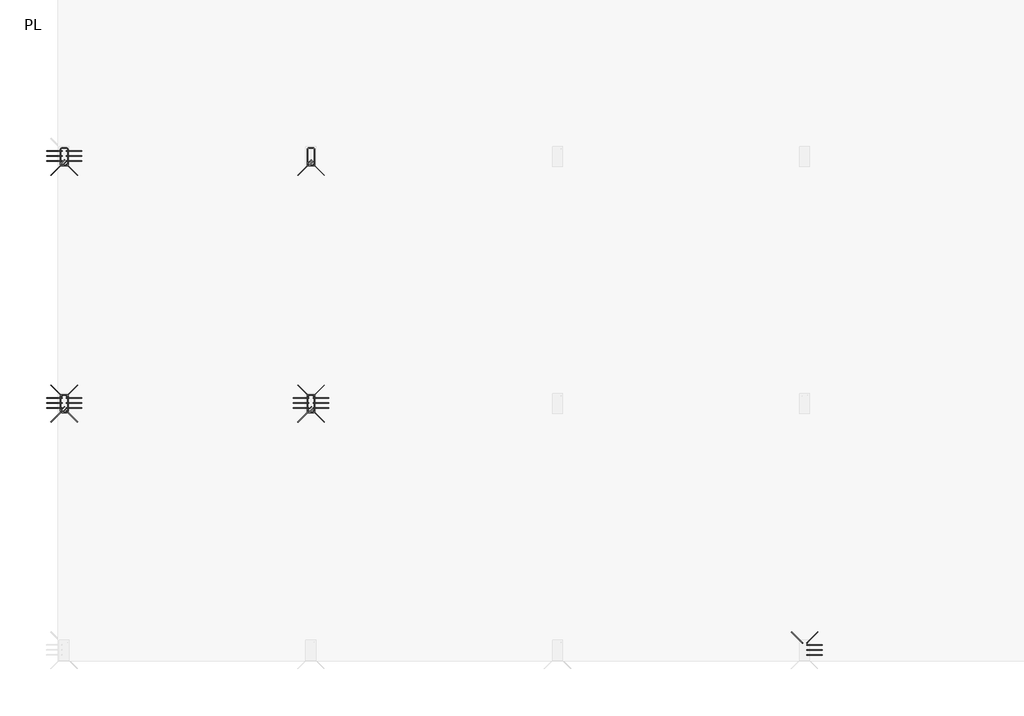
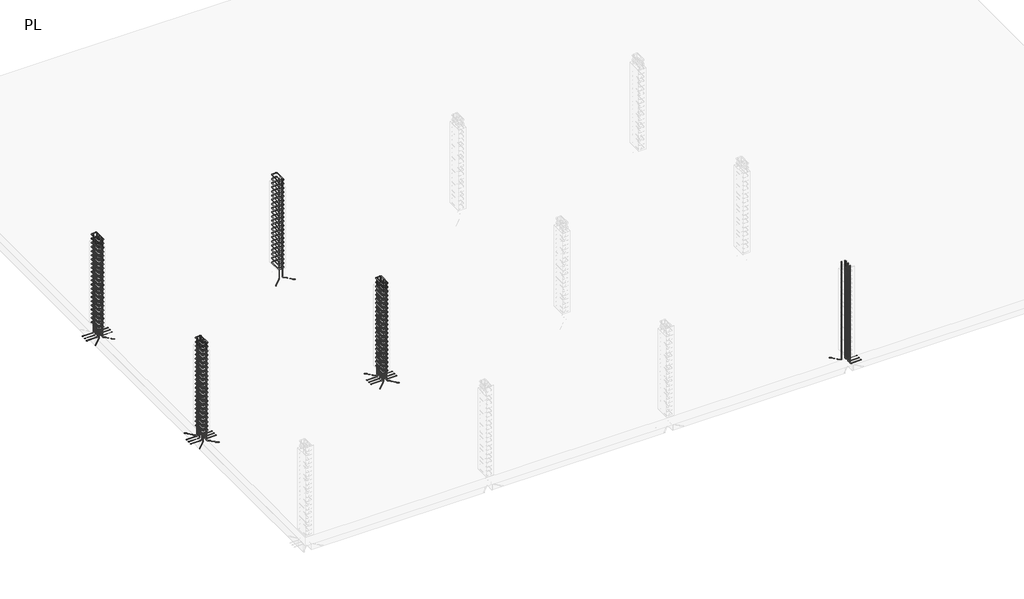
# One storey, part 4 of 10: 25 reinforcing bars.
"""IFC4 building model written with IfcOpenShell, lengths in millimetres."""

from ifc_helpers import new_model, si_unit, point, frame, origin, place, context, project, spatial, polyline, circle_curve, trimmed, segment, composite_curve, source, transform, mapped, element, save
from ifc_brep_helpers import swept_disk

model = new_model("IFC4")

# Units and contexts
model_context = context("Model", 3, world=origin())
ifc_project = project(units=[si_unit("LENGTHUNIT", "METRE", prefix="MILLI")], contexts=[model_context])

# Site, building, storey
site = spatial("IfcSite", under=ifc_project)
building = spatial("IfcBuilding", under=site)
storey = spatial("IfcBuildingStorey", under=building, Name="PL", Elevation=271.0)

# Reinforcing bars
placement = place(None, origin())
reinforcing_bar_shape = source(origin(), model_context, "Body", "SolidModel", [
    swept_disk(composite_curve([segment(polyline([(-16703.4864005, -8162.2223078, 301.0), (-16791.1676414, -8249.9035486, 301.0)]), True, "CONTINUOUS"), segment(trimmed(circle_curve(frame((-16769.9544379, -8271.1167521, 301.0), z_axis=(0.0, 0.0, 1.0), x_axis=(-21.21320349999951, 21.213203500001327, 0.0)), 30.0), [point((-16791.1676414, -8249.9035486, 301.0))], [point((-16769.9544379, -8301.1167521, 301.0))], True, "CARTESIAN"), True, "CONTINUOUS"), segment(polyline([(-16769.9544379, -8301.1167521, 301.0), (-16651.9544379, -8301.1167521, 301.0)]), True, "CONTINUOUS"), segment(trimmed(circle_curve(frame((-16651.9544379, -8271.1167521, 301.0), z_axis=(0.0, 0.0, 1.0), x_axis=(0.0, -30.0, 0.0)), 30.0), [point((-16651.9544379, -8301.1167521, 301.0))], [point((-16621.9544379, -8271.1167521, 301.0))], True, "CARTESIAN"), True, "CONTINUOUS"), segment(polyline([(-16621.9544379, -8271.1167521, 301.0), (-16621.9544379, -7903.1167521, 301.0)]), True, "CONTINUOUS"), segment(trimmed(circle_curve(frame((-16651.8864962, -7903.1167521, 298.9821084), z_axis=(-0.06726305234213417, 0.0, 0.9977352764083365), x_axis=(29.93205830000079, 0.0, 2.0178915999999845)), 30.0), [point((-16621.9544379, -7903.1167521, 301.0))], [point((-16651.8864962, -7873.1167521, 298.9821084))], True, "CARTESIAN"), True, "CONTINUOUS"), segment(polyline([(-16651.8864962, -7873.1167521, 298.9821084), (-16770.0223796, -7873.1167521, 291.0178916)]), True, "CONTINUOUS"), segment(trimmed(circle_curve(frame((-16770.0223796, -7903.1167521, 291.0178916), z_axis=(-0.06726305234213417, 0.0, 0.9977352764083365), x_axis=(0.0, 30.0, 0.0)), 30.0), [point((-16770.0223796, -7873.1167521, 291.0178916))], [point((-16799.9544379, -7903.1167521, 289.0))], True, "CARTESIAN"), True, "CONTINUOUS"), segment(polyline([(-16799.9544379, -7903.1167521, 289.0), (-16799.9544379, -8271.1167521, 289.0)]), True, "CONTINUOUS"), segment(trimmed(circle_curve(frame((-16769.9544379, -8271.1167521, 289.0), z_axis=(0.0, 0.0, 1.0), x_axis=(-30.0, 0.0, 0.0)), 30.0), [point((-16799.9544379, -8271.1167521, 289.0))], [point((-16748.7412345, -8292.3299555, 289.0))], True, "CARTESIAN"), True, "CONTINUOUS"), segment(polyline([(-16748.7412345, -8292.3299555, 289.0), (-16661.0599936, -8204.6487146, 289.0)]), True, "CONTINUOUS")], self_intersect=False), 6.0),
])
element("IfcReinforcingBar", 1, at=placement, inside=storey, context=model_context, shape_type="MappedRepresentation", body=[
    mapped(reinforcing_bar_shape, transform((0.0, 0.0, 0.0), x_axis=(1.0, 0.0, 0.0), y_axis=(0.0, 1.0, 0.0), z_axis=(0.0, 0.0, 1.0))),
    mapped(reinforcing_bar_shape, transform((0.0, 0.0, 149.2571429), x_axis=(1.0, 0.0, 0.0), y_axis=(0.0, 1.0, 0.0), z_axis=(0.0, 0.0, 1.0))),
    mapped(reinforcing_bar_shape, transform((0.0, 0.0, 298.5142857), x_axis=(1.0, 0.0, 0.0), y_axis=(0.0, 1.0, 0.0), z_axis=(0.0, 0.0, 1.0))),
    mapped(reinforcing_bar_shape, transform((0.0, 0.0, 447.7714286), x_axis=(1.0, 0.0, 0.0), y_axis=(0.0, 1.0, 0.0), z_axis=(0.0, 0.0, 1.0))),
    mapped(reinforcing_bar_shape, transform((0.0, 0.0, 597.0285714), x_axis=(1.0, 0.0, 0.0), y_axis=(0.0, 1.0, 0.0), z_axis=(0.0, 0.0, 1.0))),
    mapped(reinforcing_bar_shape, transform((0.0, 0.0, 746.2857143), x_axis=(1.0, 0.0, 0.0), y_axis=(0.0, 1.0, 0.0), z_axis=(0.0, 0.0, 1.0))),
    mapped(reinforcing_bar_shape, transform((0.0, 0.0, 895.5428571), x_axis=(1.0, 0.0, 0.0), y_axis=(0.0, 1.0, 0.0), z_axis=(0.0, 0.0, 1.0))),
    mapped(reinforcing_bar_shape, transform((0.0, 0.0, 1044.8), x_axis=(1.0, 0.0, 0.0), y_axis=(0.0, 1.0, 0.0), z_axis=(0.0, 0.0, 1.0))),
    mapped(reinforcing_bar_shape, transform((0.0, 0.0, 1194.0571429), x_axis=(1.0, 0.0, 0.0), y_axis=(0.0, 1.0, 0.0), z_axis=(0.0, 0.0, 1.0))),
    mapped(reinforcing_bar_shape, transform((0.0, 0.0, 1343.3142857), x_axis=(1.0, 0.0, 0.0), y_axis=(0.0, 1.0, 0.0), z_axis=(0.0, 0.0, 1.0))),
    mapped(reinforcing_bar_shape, transform((0.0, 0.0, 1492.5714286), x_axis=(1.0, 0.0, 0.0), y_axis=(0.0, 1.0, 0.0), z_axis=(0.0, 0.0, 1.0))),
    mapped(reinforcing_bar_shape, transform((0.0, 0.0, 1641.8285714), x_axis=(1.0, 0.0, 0.0), y_axis=(0.0, 1.0, 0.0), z_axis=(0.0, 0.0, 1.0))),
    mapped(reinforcing_bar_shape, transform((0.0, 0.0, 1791.0857143), x_axis=(1.0, 0.0, 0.0), y_axis=(0.0, 1.0, 0.0), z_axis=(0.0, 0.0, 1.0))),
    mapped(reinforcing_bar_shape, transform((0.0, 0.0, 1940.3428571), x_axis=(1.0, 0.0, 0.0), y_axis=(0.0, 1.0, 0.0), z_axis=(0.0, 0.0, 1.0))),
    mapped(reinforcing_bar_shape, transform((0.0, 0.0, 2089.6), x_axis=(1.0, 0.0, 0.0), y_axis=(0.0, 1.0, 0.0), z_axis=(0.0, 0.0, 1.0))),
    mapped(reinforcing_bar_shape, transform((0.0, 0.0, 2238.8571429), x_axis=(1.0, 0.0, 0.0), y_axis=(0.0, 1.0, 0.0), z_axis=(0.0, 0.0, 1.0))),
    mapped(reinforcing_bar_shape, transform((0.0, 0.0, 2388.1142857), x_axis=(1.0, 0.0, 0.0), y_axis=(0.0, 1.0, 0.0), z_axis=(0.0, 0.0, 1.0))),
    mapped(reinforcing_bar_shape, transform((0.0, 0.0, 2537.3714286), x_axis=(1.0, 0.0, 0.0), y_axis=(0.0, 1.0, 0.0), z_axis=(0.0, 0.0, 1.0))),
    mapped(reinforcing_bar_shape, transform((0.0, 0.0, 2686.6285714), x_axis=(1.0, 0.0, 0.0), y_axis=(0.0, 1.0, 0.0), z_axis=(0.0, 0.0, 1.0))),
    mapped(reinforcing_bar_shape, transform((0.0, 0.0, 2835.8857143), x_axis=(1.0, 0.0, 0.0), y_axis=(0.0, 1.0, 0.0), z_axis=(0.0, 0.0, 1.0))),
    mapped(reinforcing_bar_shape, transform((0.0, 0.0, 2985.1428571), x_axis=(1.0, 0.0, 0.0), y_axis=(0.0, 1.0, 0.0), z_axis=(0.0, 0.0, 1.0))),
    mapped(reinforcing_bar_shape, transform((0.0, 0.0, 3134.4), x_axis=(1.0, 0.0, 0.0), y_axis=(0.0, 1.0, 0.0), z_axis=(0.0, 0.0, 1.0))),
])
element("IfcReinforcingBar", 2, at=placement, inside=storey, context=model_context, shape_type="SolidModel", body=[
    swept_disk(composite_curve([segment(polyline([(-16768.0642232, -8272.0642439, 3441.4), (-16768.0642232, -8272.0642439, -35.0)]), True, "CONTINUOUS"), segment(trimmed(circle_curve(frame((-16789.2774266, -8293.2774473, -35.0), z_axis=(-0.7071067811865187, 0.7071067811865764, 0.0), x_axis=(21.213203400002385, 21.213203400000566, 0.0)), 30.0), [point((-16768.0642232, -8272.0642439, -35.0))], [point((-16789.2774266, -8293.2774473, -65.0))], True, "CARTESIAN"), True, "CONTINUOUS"), segment(polyline([(-16789.2774266, -8293.2774473, -65.0), (-17036.7648, -8540.7648207, -65.0)]), True, "CONTINUOUS")], self_intersect=False), 6.0),
])
element("IfcReinforcingBar", 3, at=placement, inside=storey, context=model_context, shape_type="SolidModel", body=[
    swept_disk(composite_curve([segment(polyline([(-16653.8446527, -8272.0642439, 3441.4), (-16653.8446527, -8272.0642439, -35.0)]), True, "CONTINUOUS"), segment(trimmed(circle_curve(frame((-16632.6314492, -8293.2774473, -35.0), z_axis=(-0.7071067811865248, -0.7071067811865703, 0.0), x_axis=(-21.213203500003146, 21.213203400000566, 0.0)), 30.0), [point((-16653.8446527, -8272.0642439, -35.0))], [point((-16632.6314492, -8293.2774473, -65.0))], True, "CARTESIAN"), True, "CONTINUOUS"), segment(polyline([(-16632.6314492, -8293.2774473, -65.0), (-16385.1440758, -8540.7648207, -65.0)]), True, "CONTINUOUS")], self_intersect=False), 6.0),
])
reinforcing_bar_2_shape = source(origin(), model_context, "Body", "SolidModel", [
    swept_disk(composite_curve([segment(polyline([(-22799.4864005, -8162.2223078, 301.0), (-22887.1676414, -8249.9035486, 301.0)]), True, "CONTINUOUS"), segment(trimmed(circle_curve(frame((-22865.9544379, -8271.1167521, 301.0), z_axis=(0.0, 0.0, 1.0), x_axis=(-21.21320349999951, 21.213203500001327, 0.0)), 30.0), [point((-22887.1676414, -8249.9035486, 301.0))], [point((-22865.9544379, -8301.1167521, 301.0))], True, "CARTESIAN"), True, "CONTINUOUS"), segment(polyline([(-22865.9544379, -8301.1167521, 301.0), (-22747.9544379, -8301.1167521, 301.0)]), True, "CONTINUOUS"), segment(trimmed(circle_curve(frame((-22747.9544379, -8271.1167521, 301.0), z_axis=(0.0, 0.0, 1.0), x_axis=(0.0, -30.0, 0.0)), 30.0), [point((-22747.9544379, -8301.1167521, 301.0))], [point((-22717.9544379, -8271.1167521, 301.0))], True, "CARTESIAN"), True, "CONTINUOUS"), segment(polyline([(-22717.9544379, -8271.1167521, 301.0), (-22717.9544379, -7903.1167521, 301.0)]), True, "CONTINUOUS"), segment(trimmed(circle_curve(frame((-22747.8864962, -7903.1167521, 298.9821084), z_axis=(-0.06726305234213417, 0.0, 0.9977352764083365), x_axis=(29.93205830000079, 0.0, 2.0178915999999845)), 30.0), [point((-22717.9544379, -7903.1167521, 301.0))], [point((-22747.8864962, -7873.1167521, 298.9821084))], True, "CARTESIAN"), True, "CONTINUOUS"), segment(polyline([(-22747.8864962, -7873.1167521, 298.9821084), (-22866.0223796, -7873.1167521, 291.0178916)]), True, "CONTINUOUS"), segment(trimmed(circle_curve(frame((-22866.0223796, -7903.1167521, 291.0178916), z_axis=(-0.06726305234213417, 0.0, 0.9977352764083365), x_axis=(0.0, 30.0, 0.0)), 30.0), [point((-22866.0223796, -7873.1167521, 291.0178916))], [point((-22895.9544379, -7903.1167521, 289.0))], True, "CARTESIAN"), True, "CONTINUOUS"), segment(polyline([(-22895.9544379, -7903.1167521, 289.0), (-22895.9544379, -8271.1167521, 289.0)]), True, "CONTINUOUS"), segment(trimmed(circle_curve(frame((-22865.9544379, -8271.1167521, 289.0), z_axis=(0.0, 0.0, 1.0), x_axis=(-30.0, 0.0, 0.0)), 30.0), [point((-22895.9544379, -8271.1167521, 289.0))], [point((-22844.7412345, -8292.3299555, 289.0))], True, "CARTESIAN"), True, "CONTINUOUS"), segment(polyline([(-22844.7412345, -8292.3299555, 289.0), (-22757.0599936, -8204.6487146, 289.0)]), True, "CONTINUOUS")], self_intersect=False), 6.0),
])
element("IfcReinforcingBar", 4, at=placement, inside=storey, context=model_context, shape_type="MappedRepresentation", body=[
    mapped(reinforcing_bar_2_shape, transform((0.0, 0.0, 0.0), x_axis=(1.0, 0.0, 0.0), y_axis=(0.0, 1.0, 0.0), z_axis=(0.0, 0.0, 1.0))),
    mapped(reinforcing_bar_2_shape, transform((0.0, 0.0, 149.2571429), x_axis=(1.0, 0.0, 0.0), y_axis=(0.0, 1.0, 0.0), z_axis=(0.0, 0.0, 1.0))),
    mapped(reinforcing_bar_2_shape, transform((0.0, 0.0, 298.5142857), x_axis=(1.0, 0.0, 0.0), y_axis=(0.0, 1.0, 0.0), z_axis=(0.0, 0.0, 1.0))),
    mapped(reinforcing_bar_2_shape, transform((0.0, 0.0, 447.7714286), x_axis=(1.0, 0.0, 0.0), y_axis=(0.0, 1.0, 0.0), z_axis=(0.0, 0.0, 1.0))),
    mapped(reinforcing_bar_2_shape, transform((0.0, 0.0, 597.0285714), x_axis=(1.0, 0.0, 0.0), y_axis=(0.0, 1.0, 0.0), z_axis=(0.0, 0.0, 1.0))),
    mapped(reinforcing_bar_2_shape, transform((0.0, 0.0, 746.2857143), x_axis=(1.0, 0.0, 0.0), y_axis=(0.0, 1.0, 0.0), z_axis=(0.0, 0.0, 1.0))),
    mapped(reinforcing_bar_2_shape, transform((0.0, 0.0, 895.5428571), x_axis=(1.0, 0.0, 0.0), y_axis=(0.0, 1.0, 0.0), z_axis=(0.0, 0.0, 1.0))),
    mapped(reinforcing_bar_2_shape, transform((0.0, 0.0, 1044.8), x_axis=(1.0, 0.0, 0.0), y_axis=(0.0, 1.0, 0.0), z_axis=(0.0, 0.0, 1.0))),
    mapped(reinforcing_bar_2_shape, transform((0.0, 0.0, 1194.0571429), x_axis=(1.0, 0.0, 0.0), y_axis=(0.0, 1.0, 0.0), z_axis=(0.0, 0.0, 1.0))),
    mapped(reinforcing_bar_2_shape, transform((0.0, 0.0, 1343.3142857), x_axis=(1.0, 0.0, 0.0), y_axis=(0.0, 1.0, 0.0), z_axis=(0.0, 0.0, 1.0))),
    mapped(reinforcing_bar_2_shape, transform((0.0, 0.0, 1492.5714286), x_axis=(1.0, 0.0, 0.0), y_axis=(0.0, 1.0, 0.0), z_axis=(0.0, 0.0, 1.0))),
    mapped(reinforcing_bar_2_shape, transform((0.0, 0.0, 1641.8285714), x_axis=(1.0, 0.0, 0.0), y_axis=(0.0, 1.0, 0.0), z_axis=(0.0, 0.0, 1.0))),
    mapped(reinforcing_bar_2_shape, transform((0.0, 0.0, 1791.0857143), x_axis=(1.0, 0.0, 0.0), y_axis=(0.0, 1.0, 0.0), z_axis=(0.0, 0.0, 1.0))),
    mapped(reinforcing_bar_2_shape, transform((0.0, 0.0, 1940.3428571), x_axis=(1.0, 0.0, 0.0), y_axis=(0.0, 1.0, 0.0), z_axis=(0.0, 0.0, 1.0))),
    mapped(reinforcing_bar_2_shape, transform((0.0, 0.0, 2089.6), x_axis=(1.0, 0.0, 0.0), y_axis=(0.0, 1.0, 0.0), z_axis=(0.0, 0.0, 1.0))),
    mapped(reinforcing_bar_2_shape, transform((0.0, 0.0, 2238.8571429), x_axis=(1.0, 0.0, 0.0), y_axis=(0.0, 1.0, 0.0), z_axis=(0.0, 0.0, 1.0))),
    mapped(reinforcing_bar_2_shape, transform((0.0, 0.0, 2388.1142857), x_axis=(1.0, 0.0, 0.0), y_axis=(0.0, 1.0, 0.0), z_axis=(0.0, 0.0, 1.0))),
    mapped(reinforcing_bar_2_shape, transform((0.0, 0.0, 2537.3714286), x_axis=(1.0, 0.0, 0.0), y_axis=(0.0, 1.0, 0.0), z_axis=(0.0, 0.0, 1.0))),
    mapped(reinforcing_bar_2_shape, transform((0.0, 0.0, 2686.6285714), x_axis=(1.0, 0.0, 0.0), y_axis=(0.0, 1.0, 0.0), z_axis=(0.0, 0.0, 1.0))),
    mapped(reinforcing_bar_2_shape, transform((0.0, 0.0, 2835.8857143), x_axis=(1.0, 0.0, 0.0), y_axis=(0.0, 1.0, 0.0), z_axis=(0.0, 0.0, 1.0))),
    mapped(reinforcing_bar_2_shape, transform((0.0, 0.0, 2985.1428571), x_axis=(1.0, 0.0, 0.0), y_axis=(0.0, 1.0, 0.0), z_axis=(0.0, 0.0, 1.0))),
    mapped(reinforcing_bar_2_shape, transform((0.0, 0.0, 3134.4), x_axis=(1.0, 0.0, 0.0), y_axis=(0.0, 1.0, 0.0), z_axis=(0.0, 0.0, 1.0))),
])
element("IfcReinforcingBar", 5, at=placement, inside=storey, context=model_context, shape_type="SolidModel", body=[
    swept_disk(composite_curve([segment(polyline([(-22864.0642232, -8272.0642439, 3441.4), (-22864.0642232, -8272.0642439, -35.0)]), True, "CONTINUOUS"), segment(trimmed(circle_curve(frame((-22885.2774266, -8293.2774473, -35.0), z_axis=(-0.7071067811865187, 0.7071067811865764, 0.0), x_axis=(21.213203400002385, 21.213203400000566, 0.0)), 30.0), [point((-22864.0642232, -8272.0642439, -35.0))], [point((-22885.2774266, -8293.2774473, -65.0))], True, "CARTESIAN"), True, "CONTINUOUS"), segment(polyline([(-22885.2774266, -8293.2774473, -65.0), (-23132.7648, -8540.7648207, -65.0)]), True, "CONTINUOUS")], self_intersect=False), 6.0),
])
element("IfcReinforcingBar", 6, at=placement, inside=storey, context=model_context, shape_type="SolidModel", body=[
    swept_disk(composite_curve([segment(polyline([(-22749.8446527, -8272.0642439, 3441.4), (-22749.8446527, -8272.0642439, -35.0)]), True, "CONTINUOUS"), segment(trimmed(circle_curve(frame((-22728.6314492, -8293.2774473, -35.0), z_axis=(-0.7071067811865248, -0.7071067811865703, 0.0), x_axis=(-21.213203500003146, 21.213203400000566, 0.0)), 30.0), [point((-22749.8446527, -8272.0642439, -35.0))], [point((-22728.6314492, -8293.2774473, -65.0))], True, "CARTESIAN"), True, "CONTINUOUS"), segment(polyline([(-22728.6314492, -8293.2774473, -65.0), (-22481.1440758, -8540.7648207, -65.0)]), True, "CONTINUOUS")], self_intersect=False), 6.0),
])
reinforcing_bar_3_shape = source(origin(), model_context, "Body", "SolidModel", [
    swept_disk(composite_curve([segment(polyline([(-22864.0642232, -8194.9117405, 3441.4), (-22864.0642232, -8194.9117405, -35.0)]), True, "CONTINUOUS"), segment(trimmed(circle_curve(frame((-22894.0642232, -8194.9117405, -35.0), z_axis=(0.0, 1.0, 0.0), x_axis=(30.0, 0.0, 0.0)), 30.0), [point((-22864.0642232, -8194.9117405, -35.0))], [point((-22894.0642232, -8194.9117405, -65.0))], True, "CARTESIAN"), True, "CONTINUOUS"), segment(polyline([(-22894.0642232, -8194.9117405, -65.0), (-23244.0642232, -8194.9117405, -65.0)]), True, "CONTINUOUS")], self_intersect=False), 6.0),
])
element("IfcReinforcingBar", 7, at=placement, inside=storey, context=model_context, shape_type="MappedRepresentation", body=[
    mapped(reinforcing_bar_3_shape, transform((0.0, 0.0, 0.0), x_axis=(1.0, 0.0, 0.0), y_axis=(0.0, 1.0, 0.0), z_axis=(0.0, 0.0, 1.0))),
    mapped(reinforcing_bar_3_shape, transform((0.0, 123.5823926, 0.0), x_axis=(1.0, 0.0, 0.0), y_axis=(0.0, 1.0, 0.0), z_axis=(0.0, 0.0, 1.0))),
    mapped(reinforcing_bar_3_shape, transform((0.0, 247.1647853, 0.0), x_axis=(1.0, 0.0, 0.0), y_axis=(0.0, 1.0, 0.0), z_axis=(0.0, 0.0, 1.0))),
])
reinforcing_bar_4_shape = source(origin(), model_context, "Body", "SolidModel", [
    swept_disk(composite_curve([segment(polyline([(-22749.8446527, -8194.9117405, 3441.4), (-22749.8446527, -8194.9117405, -35.0)]), True, "CONTINUOUS"), segment(trimmed(circle_curve(frame((-22719.8446527, -8194.9117405, -35.0), z_axis=(0.0, -1.0, 0.0), x_axis=(-30.0, 0.0, 0.0)), 30.0), [point((-22749.8446527, -8194.9117405, -35.0))], [point((-22719.8446527, -8194.9117405, -65.0))], True, "CARTESIAN"), True, "CONTINUOUS"), segment(polyline([(-22719.8446527, -8194.9117405, -65.0), (-22369.8446527, -8194.9117405, -65.0)]), True, "CONTINUOUS")], self_intersect=False), 6.0),
])
element("IfcReinforcingBar", 8, at=placement, inside=storey, context=model_context, shape_type="MappedRepresentation", body=[
    mapped(reinforcing_bar_4_shape, transform((0.0, 0.0, 0.0), x_axis=(1.0, 0.0, 0.0), y_axis=(0.0, 1.0, 0.0), z_axis=(0.0, 0.0, 1.0))),
    mapped(reinforcing_bar_4_shape, transform((0.0, 123.5823926, 0.0), x_axis=(1.0, 0.0, 0.0), y_axis=(0.0, 1.0, 0.0), z_axis=(0.0, 0.0, 1.0))),
    mapped(reinforcing_bar_4_shape, transform((0.0, 247.1647853, 0.0), x_axis=(1.0, 0.0, 0.0), y_axis=(0.0, 1.0, 0.0), z_axis=(0.0, 0.0, 1.0))),
])
reinforcing_bar_5_shape = source(origin(), model_context, "Body", "SolidModel", [
    swept_disk(composite_curve([segment(polyline([(-22799.4864005, -14258.2223078, 301.0), (-22887.1676414, -14345.9035486, 301.0)]), True, "CONTINUOUS"), segment(trimmed(circle_curve(frame((-22865.9544379, -14367.1167521, 301.0), z_axis=(0.0, 0.0, 1.0), x_axis=(-21.21320349999951, 21.213203500001327, 0.0)), 30.0), [point((-22887.1676414, -14345.9035486, 301.0))], [point((-22865.9544379, -14397.1167521, 301.0))], True, "CARTESIAN"), True, "CONTINUOUS"), segment(polyline([(-22865.9544379, -14397.1167521, 301.0), (-22747.9544379, -14397.1167521, 301.0)]), True, "CONTINUOUS"), segment(trimmed(circle_curve(frame((-22747.9544379, -14367.1167521, 301.0), z_axis=(0.0, 0.0, 1.0), x_axis=(0.0, -30.0, 0.0)), 30.0), [point((-22747.9544379, -14397.1167521, 301.0))], [point((-22717.9544379, -14367.1167521, 301.0))], True, "CARTESIAN"), True, "CONTINUOUS"), segment(polyline([(-22717.9544379, -14367.1167521, 301.0), (-22717.9544379, -13999.1167521, 301.0)]), True, "CONTINUOUS"), segment(trimmed(circle_curve(frame((-22747.8864962, -13999.1167521, 298.9821084), z_axis=(-0.06726305234213417, 0.0, 0.9977352764083365), x_axis=(29.93205830000079, 0.0, 2.0178915999999845)), 30.0), [point((-22717.9544379, -13999.1167521, 301.0))], [point((-22747.8864962, -13969.1167521, 298.9821084))], True, "CARTESIAN"), True, "CONTINUOUS"), segment(polyline([(-22747.8864962, -13969.1167521, 298.9821084), (-22866.0223796, -13969.1167521, 291.0178916)]), True, "CONTINUOUS"), segment(trimmed(circle_curve(frame((-22866.0223796, -13999.1167521, 291.0178916), z_axis=(-0.06726305234213417, 0.0, 0.9977352764083365), x_axis=(0.0, 30.0, 0.0)), 30.0), [point((-22866.0223796, -13969.1167521, 291.0178916))], [point((-22895.9544379, -13999.1167521, 289.0))], True, "CARTESIAN"), True, "CONTINUOUS"), segment(polyline([(-22895.9544379, -13999.1167521, 289.0), (-22895.9544379, -14367.1167521, 289.0)]), True, "CONTINUOUS"), segment(trimmed(circle_curve(frame((-22865.9544379, -14367.1167521, 289.0), z_axis=(0.0, 0.0, 1.0), x_axis=(-30.0, 0.0, 0.0)), 30.0), [point((-22895.9544379, -14367.1167521, 289.0))], [point((-22844.7412345, -14388.3299555, 289.0))], True, "CARTESIAN"), True, "CONTINUOUS"), segment(polyline([(-22844.7412345, -14388.3299555, 289.0), (-22757.0599936, -14300.6487146, 289.0)]), True, "CONTINUOUS")], self_intersect=False), 6.0),
])
element("IfcReinforcingBar", 9, at=placement, inside=storey, context=model_context, shape_type="MappedRepresentation", body=[
    mapped(reinforcing_bar_5_shape, transform((0.0, 0.0, 0.0), x_axis=(1.0, 0.0, 0.0), y_axis=(0.0, 1.0, 0.0), z_axis=(0.0, 0.0, 1.0))),
    mapped(reinforcing_bar_5_shape, transform((0.0, 0.0, 149.2571429), x_axis=(1.0, 0.0, 0.0), y_axis=(0.0, 1.0, 0.0), z_axis=(0.0, 0.0, 1.0))),
    mapped(reinforcing_bar_5_shape, transform((0.0, 0.0, 298.5142857), x_axis=(1.0, 0.0, 0.0), y_axis=(0.0, 1.0, 0.0), z_axis=(0.0, 0.0, 1.0))),
    mapped(reinforcing_bar_5_shape, transform((0.0, 0.0, 447.7714286), x_axis=(1.0, 0.0, 0.0), y_axis=(0.0, 1.0, 0.0), z_axis=(0.0, 0.0, 1.0))),
    mapped(reinforcing_bar_5_shape, transform((0.0, 0.0, 597.0285714), x_axis=(1.0, 0.0, 0.0), y_axis=(0.0, 1.0, 0.0), z_axis=(0.0, 0.0, 1.0))),
    mapped(reinforcing_bar_5_shape, transform((0.0, 0.0, 746.2857143), x_axis=(1.0, 0.0, 0.0), y_axis=(0.0, 1.0, 0.0), z_axis=(0.0, 0.0, 1.0))),
    mapped(reinforcing_bar_5_shape, transform((0.0, 0.0, 895.5428571), x_axis=(1.0, 0.0, 0.0), y_axis=(0.0, 1.0, 0.0), z_axis=(0.0, 0.0, 1.0))),
    mapped(reinforcing_bar_5_shape, transform((0.0, 0.0, 1044.8), x_axis=(1.0, 0.0, 0.0), y_axis=(0.0, 1.0, 0.0), z_axis=(0.0, 0.0, 1.0))),
    mapped(reinforcing_bar_5_shape, transform((0.0, 0.0, 1194.0571429), x_axis=(1.0, 0.0, 0.0), y_axis=(0.0, 1.0, 0.0), z_axis=(0.0, 0.0, 1.0))),
    mapped(reinforcing_bar_5_shape, transform((0.0, 0.0, 1343.3142857), x_axis=(1.0, 0.0, 0.0), y_axis=(0.0, 1.0, 0.0), z_axis=(0.0, 0.0, 1.0))),
    mapped(reinforcing_bar_5_shape, transform((0.0, 0.0, 1492.5714286), x_axis=(1.0, 0.0, 0.0), y_axis=(0.0, 1.0, 0.0), z_axis=(0.0, 0.0, 1.0))),
    mapped(reinforcing_bar_5_shape, transform((0.0, 0.0, 1641.8285714), x_axis=(1.0, 0.0, 0.0), y_axis=(0.0, 1.0, 0.0), z_axis=(0.0, 0.0, 1.0))),
    mapped(reinforcing_bar_5_shape, transform((0.0, 0.0, 1791.0857143), x_axis=(1.0, 0.0, 0.0), y_axis=(0.0, 1.0, 0.0), z_axis=(0.0, 0.0, 1.0))),
    mapped(reinforcing_bar_5_shape, transform((0.0, 0.0, 1940.3428571), x_axis=(1.0, 0.0, 0.0), y_axis=(0.0, 1.0, 0.0), z_axis=(0.0, 0.0, 1.0))),
    mapped(reinforcing_bar_5_shape, transform((0.0, 0.0, 2089.6), x_axis=(1.0, 0.0, 0.0), y_axis=(0.0, 1.0, 0.0), z_axis=(0.0, 0.0, 1.0))),
    mapped(reinforcing_bar_5_shape, transform((0.0, 0.0, 2238.8571429), x_axis=(1.0, 0.0, 0.0), y_axis=(0.0, 1.0, 0.0), z_axis=(0.0, 0.0, 1.0))),
    mapped(reinforcing_bar_5_shape, transform((0.0, 0.0, 2388.1142857), x_axis=(1.0, 0.0, 0.0), y_axis=(0.0, 1.0, 0.0), z_axis=(0.0, 0.0, 1.0))),
    mapped(reinforcing_bar_5_shape, transform((0.0, 0.0, 2537.3714286), x_axis=(1.0, 0.0, 0.0), y_axis=(0.0, 1.0, 0.0), z_axis=(0.0, 0.0, 1.0))),
    mapped(reinforcing_bar_5_shape, transform((0.0, 0.0, 2686.6285714), x_axis=(1.0, 0.0, 0.0), y_axis=(0.0, 1.0, 0.0), z_axis=(0.0, 0.0, 1.0))),
    mapped(reinforcing_bar_5_shape, transform((0.0, 0.0, 2835.8857143), x_axis=(1.0, 0.0, 0.0), y_axis=(0.0, 1.0, 0.0), z_axis=(0.0, 0.0, 1.0))),
    mapped(reinforcing_bar_5_shape, transform((0.0, 0.0, 2985.1428571), x_axis=(1.0, 0.0, 0.0), y_axis=(0.0, 1.0, 0.0), z_axis=(0.0, 0.0, 1.0))),
    mapped(reinforcing_bar_5_shape, transform((0.0, 0.0, 3134.4), x_axis=(1.0, 0.0, 0.0), y_axis=(0.0, 1.0, 0.0), z_axis=(0.0, 0.0, 1.0))),
])
element("IfcReinforcingBar", 10, at=placement, inside=storey, context=model_context, shape_type="SolidModel", body=[
    swept_disk(composite_curve([segment(polyline([(-22864.0642232, -14368.0642439, 3441.4), (-22864.0642232, -14368.0642439, -35.0)]), True, "CONTINUOUS"), segment(trimmed(circle_curve(frame((-22885.2774266, -14389.2774473, -35.0), z_axis=(-0.7071067811865187, 0.7071067811865764, 0.0), x_axis=(21.213203400002385, 21.213203400000566, 0.0)), 30.0), [point((-22864.0642232, -14368.0642439, -35.0))], [point((-22885.2774266, -14389.2774473, -65.0))], True, "CARTESIAN"), True, "CONTINUOUS"), segment(polyline([(-22885.2774266, -14389.2774473, -65.0), (-23132.7648, -14636.7648207, -65.0)]), True, "CONTINUOUS")], self_intersect=False), 6.0),
])
element("IfcReinforcingBar", 11, at=placement, inside=storey, context=model_context, shape_type="SolidModel", body=[
    swept_disk(composite_curve([segment(polyline([(-22864.0642232, -13998.1692603, 3441.4), (-22864.0642232, -13998.1692603, -35.0)]), True, "CONTINUOUS"), segment(trimmed(circle_curve(frame((-22885.2774266, -13976.9560568, -35.0), z_axis=(0.7071067811865218, 0.7071067811865733, 0.0), x_axis=(21.213203400002385, -21.21320349999951, 0.0)), 30.0), [point((-22864.0642232, -13998.1692603, -35.0))], [point((-22885.2774266, -13976.9560568, -65.0))], True, "CARTESIAN"), True, "CONTINUOUS"), segment(polyline([(-22885.2774266, -13976.9560568, -65.0), (-23132.7648, -13729.4686834, -65.0)]), True, "CONTINUOUS")], self_intersect=False), 6.0),
])
element("IfcReinforcingBar", 12, at=placement, inside=storey, context=model_context, shape_type="SolidModel", body=[
    swept_disk(composite_curve([segment(polyline([(-22749.8446527, -14368.0642439, 3441.4), (-22749.8446527, -14368.0642439, -35.0)]), True, "CONTINUOUS"), segment(trimmed(circle_curve(frame((-22728.6314492, -14389.2774473, -35.0), z_axis=(-0.7071067811865248, -0.7071067811865703, 0.0), x_axis=(-21.213203500003146, 21.213203400000566, 0.0)), 30.0), [point((-22749.8446527, -14368.0642439, -35.0))], [point((-22728.6314492, -14389.2774473, -65.0))], True, "CARTESIAN"), True, "CONTINUOUS"), segment(polyline([(-22728.6314492, -14389.2774473, -65.0), (-22481.1440758, -14636.7648207, -65.0)]), True, "CONTINUOUS")], self_intersect=False), 6.0),
])
element("IfcReinforcingBar", 13, at=placement, inside=storey, context=model_context, shape_type="SolidModel", body=[
    swept_disk(composite_curve([segment(polyline([(-22749.8446527, -13998.1692603, 3441.4), (-22749.8446527, -13998.1692603, -35.0)]), True, "CONTINUOUS"), segment(trimmed(circle_curve(frame((-22728.6314492, -13976.9560568, -35.0), z_axis=(0.7071067811865157, -0.7071067811865794, 0.0), x_axis=(-21.213203500003146, -21.21320349999951, 0.0)), 30.0), [point((-22749.8446527, -13998.1692603, -35.0))], [point((-22728.6314492, -13976.9560568, -65.0))], True, "CARTESIAN"), True, "CONTINUOUS"), segment(polyline([(-22728.6314492, -13976.9560568, -65.0), (-22481.1440758, -13729.4686834, -65.0)]), True, "CONTINUOUS")], self_intersect=False), 6.0),
])
reinforcing_bar_6_shape = source(origin(), model_context, "Body", "SolidModel", [
    swept_disk(composite_curve([segment(polyline([(-22864.0642232, -14290.9117405, 3441.4), (-22864.0642232, -14290.9117405, -35.0)]), True, "CONTINUOUS"), segment(trimmed(circle_curve(frame((-22894.0642232, -14290.9117405, -35.0), z_axis=(0.0, 1.0, 0.0), x_axis=(30.0, 0.0, 0.0)), 30.0), [point((-22864.0642232, -14290.9117405, -35.0))], [point((-22894.0642232, -14290.9117405, -65.0))], True, "CARTESIAN"), True, "CONTINUOUS"), segment(polyline([(-22894.0642232, -14290.9117405, -65.0), (-23244.0642232, -14290.9117405, -65.0)]), True, "CONTINUOUS")], self_intersect=False), 6.0),
])
element("IfcReinforcingBar", 14, at=placement, inside=storey, context=model_context, shape_type="MappedRepresentation", body=[
    mapped(reinforcing_bar_6_shape, transform((0.0, 0.0, 0.0), x_axis=(1.0, 0.0, 0.0), y_axis=(0.0, 1.0, 0.0), z_axis=(0.0, 0.0, 1.0))),
    mapped(reinforcing_bar_6_shape, transform((0.0, 123.5823926, 0.0), x_axis=(1.0, 0.0, 0.0), y_axis=(0.0, 1.0, 0.0), z_axis=(0.0, 0.0, 1.0))),
    mapped(reinforcing_bar_6_shape, transform((0.0, 247.1647853, 0.0), x_axis=(1.0, 0.0, 0.0), y_axis=(0.0, 1.0, 0.0), z_axis=(0.0, 0.0, 1.0))),
])
reinforcing_bar_7_shape = source(origin(), model_context, "Body", "SolidModel", [
    swept_disk(composite_curve([segment(polyline([(-22749.8446527, -14290.9117405, 3441.4), (-22749.8446527, -14290.9117405, -35.0)]), True, "CONTINUOUS"), segment(trimmed(circle_curve(frame((-22719.8446527, -14290.9117405, -35.0), z_axis=(0.0, -1.0, 0.0), x_axis=(-30.0, 0.0, 0.0)), 30.0), [point((-22749.8446527, -14290.9117405, -35.0))], [point((-22719.8446527, -14290.9117405, -65.0))], True, "CARTESIAN"), True, "CONTINUOUS"), segment(polyline([(-22719.8446527, -14290.9117405, -65.0), (-22369.8446527, -14290.9117405, -65.0)]), True, "CONTINUOUS")], self_intersect=False), 6.0),
])
element("IfcReinforcingBar", 15, at=placement, inside=storey, context=model_context, shape_type="MappedRepresentation", body=[
    mapped(reinforcing_bar_7_shape, transform((0.0, 0.0, 0.0), x_axis=(1.0, 0.0, 0.0), y_axis=(0.0, 1.0, 0.0), z_axis=(0.0, 0.0, 1.0))),
    mapped(reinforcing_bar_7_shape, transform((0.0, 123.5823926, 0.0), x_axis=(1.0, 0.0, 0.0), y_axis=(0.0, 1.0, 0.0), z_axis=(0.0, 0.0, 1.0))),
    mapped(reinforcing_bar_7_shape, transform((0.0, 247.1647853, 0.0), x_axis=(1.0, 0.0, 0.0), y_axis=(0.0, 1.0, 0.0), z_axis=(0.0, 0.0, 1.0))),
])
reinforcing_bar_8_shape = source(origin(), model_context, "Body", "SolidModel", [
    swept_disk(composite_curve([segment(polyline([(-16703.4864005, -14258.2223078, 301.0), (-16791.1676414, -14345.9035486, 301.0)]), True, "CONTINUOUS"), segment(trimmed(circle_curve(frame((-16769.9544379, -14367.1167521, 301.0), z_axis=(0.0, 0.0, 1.0), x_axis=(-21.21320349999951, 21.213203500001327, 0.0)), 30.0), [point((-16791.1676414, -14345.9035486, 301.0))], [point((-16769.9544379, -14397.1167521, 301.0))], True, "CARTESIAN"), True, "CONTINUOUS"), segment(polyline([(-16769.9544379, -14397.1167521, 301.0), (-16651.9544379, -14397.1167521, 301.0)]), True, "CONTINUOUS"), segment(trimmed(circle_curve(frame((-16651.9544379, -14367.1167521, 301.0), z_axis=(0.0, 0.0, 1.0), x_axis=(0.0, -30.0, 0.0)), 30.0), [point((-16651.9544379, -14397.1167521, 301.0))], [point((-16621.9544379, -14367.1167521, 301.0))], True, "CARTESIAN"), True, "CONTINUOUS"), segment(polyline([(-16621.9544379, -14367.1167521, 301.0), (-16621.9544379, -13999.1167521, 301.0)]), True, "CONTINUOUS"), segment(trimmed(circle_curve(frame((-16651.8864962, -13999.1167521, 298.9821084), z_axis=(-0.06726305234213417, 0.0, 0.9977352764083365), x_axis=(29.93205830000079, 0.0, 2.0178915999999845)), 30.0), [point((-16621.9544379, -13999.1167521, 301.0))], [point((-16651.8864962, -13969.1167521, 298.9821084))], True, "CARTESIAN"), True, "CONTINUOUS"), segment(polyline([(-16651.8864962, -13969.1167521, 298.9821084), (-16770.0223796, -13969.1167521, 291.0178916)]), True, "CONTINUOUS"), segment(trimmed(circle_curve(frame((-16770.0223796, -13999.1167521, 291.0178916), z_axis=(-0.06726305234213417, 0.0, 0.9977352764083365), x_axis=(0.0, 30.0, 0.0)), 30.0), [point((-16770.0223796, -13969.1167521, 291.0178916))], [point((-16799.9544379, -13999.1167521, 289.0))], True, "CARTESIAN"), True, "CONTINUOUS"), segment(polyline([(-16799.9544379, -13999.1167521, 289.0), (-16799.9544379, -14367.1167521, 289.0)]), True, "CONTINUOUS"), segment(trimmed(circle_curve(frame((-16769.9544379, -14367.1167521, 289.0), z_axis=(0.0, 0.0, 1.0), x_axis=(-30.0, 0.0, 0.0)), 30.0), [point((-16799.9544379, -14367.1167521, 289.0))], [point((-16748.7412345, -14388.3299555, 289.0))], True, "CARTESIAN"), True, "CONTINUOUS"), segment(polyline([(-16748.7412345, -14388.3299555, 289.0), (-16661.0599936, -14300.6487146, 289.0)]), True, "CONTINUOUS")], self_intersect=False), 6.0),
])
element("IfcReinforcingBar", 16, at=placement, inside=storey, context=model_context, shape_type="MappedRepresentation", body=[
    mapped(reinforcing_bar_8_shape, transform((0.0, 0.0, 0.0), x_axis=(1.0, 0.0, 0.0), y_axis=(0.0, 1.0, 0.0), z_axis=(0.0, 0.0, 1.0))),
    mapped(reinforcing_bar_8_shape, transform((0.0, 0.0, 149.2571429), x_axis=(1.0, 0.0, 0.0), y_axis=(0.0, 1.0, 0.0), z_axis=(0.0, 0.0, 1.0))),
    mapped(reinforcing_bar_8_shape, transform((0.0, 0.0, 298.5142857), x_axis=(1.0, 0.0, 0.0), y_axis=(0.0, 1.0, 0.0), z_axis=(0.0, 0.0, 1.0))),
    mapped(reinforcing_bar_8_shape, transform((0.0, 0.0, 447.7714286), x_axis=(1.0, 0.0, 0.0), y_axis=(0.0, 1.0, 0.0), z_axis=(0.0, 0.0, 1.0))),
    mapped(reinforcing_bar_8_shape, transform((0.0, 0.0, 597.0285714), x_axis=(1.0, 0.0, 0.0), y_axis=(0.0, 1.0, 0.0), z_axis=(0.0, 0.0, 1.0))),
    mapped(reinforcing_bar_8_shape, transform((0.0, 0.0, 746.2857143), x_axis=(1.0, 0.0, 0.0), y_axis=(0.0, 1.0, 0.0), z_axis=(0.0, 0.0, 1.0))),
    mapped(reinforcing_bar_8_shape, transform((0.0, 0.0, 895.5428571), x_axis=(1.0, 0.0, 0.0), y_axis=(0.0, 1.0, 0.0), z_axis=(0.0, 0.0, 1.0))),
    mapped(reinforcing_bar_8_shape, transform((0.0, 0.0, 1044.8), x_axis=(1.0, 0.0, 0.0), y_axis=(0.0, 1.0, 0.0), z_axis=(0.0, 0.0, 1.0))),
    mapped(reinforcing_bar_8_shape, transform((0.0, 0.0, 1194.0571429), x_axis=(1.0, 0.0, 0.0), y_axis=(0.0, 1.0, 0.0), z_axis=(0.0, 0.0, 1.0))),
    mapped(reinforcing_bar_8_shape, transform((0.0, 0.0, 1343.3142857), x_axis=(1.0, 0.0, 0.0), y_axis=(0.0, 1.0, 0.0), z_axis=(0.0, 0.0, 1.0))),
    mapped(reinforcing_bar_8_shape, transform((0.0, 0.0, 1492.5714286), x_axis=(1.0, 0.0, 0.0), y_axis=(0.0, 1.0, 0.0), z_axis=(0.0, 0.0, 1.0))),
    mapped(reinforcing_bar_8_shape, transform((0.0, 0.0, 1641.8285714), x_axis=(1.0, 0.0, 0.0), y_axis=(0.0, 1.0, 0.0), z_axis=(0.0, 0.0, 1.0))),
    mapped(reinforcing_bar_8_shape, transform((0.0, 0.0, 1791.0857143), x_axis=(1.0, 0.0, 0.0), y_axis=(0.0, 1.0, 0.0), z_axis=(0.0, 0.0, 1.0))),
    mapped(reinforcing_bar_8_shape, transform((0.0, 0.0, 1940.3428571), x_axis=(1.0, 0.0, 0.0), y_axis=(0.0, 1.0, 0.0), z_axis=(0.0, 0.0, 1.0))),
    mapped(reinforcing_bar_8_shape, transform((0.0, 0.0, 2089.6), x_axis=(1.0, 0.0, 0.0), y_axis=(0.0, 1.0, 0.0), z_axis=(0.0, 0.0, 1.0))),
    mapped(reinforcing_bar_8_shape, transform((0.0, 0.0, 2238.8571429), x_axis=(1.0, 0.0, 0.0), y_axis=(0.0, 1.0, 0.0), z_axis=(0.0, 0.0, 1.0))),
    mapped(reinforcing_bar_8_shape, transform((0.0, 0.0, 2388.1142857), x_axis=(1.0, 0.0, 0.0), y_axis=(0.0, 1.0, 0.0), z_axis=(0.0, 0.0, 1.0))),
    mapped(reinforcing_bar_8_shape, transform((0.0, 0.0, 2537.3714286), x_axis=(1.0, 0.0, 0.0), y_axis=(0.0, 1.0, 0.0), z_axis=(0.0, 0.0, 1.0))),
    mapped(reinforcing_bar_8_shape, transform((0.0, 0.0, 2686.6285714), x_axis=(1.0, 0.0, 0.0), y_axis=(0.0, 1.0, 0.0), z_axis=(0.0, 0.0, 1.0))),
    mapped(reinforcing_bar_8_shape, transform((0.0, 0.0, 2835.8857143), x_axis=(1.0, 0.0, 0.0), y_axis=(0.0, 1.0, 0.0), z_axis=(0.0, 0.0, 1.0))),
    mapped(reinforcing_bar_8_shape, transform((0.0, 0.0, 2985.1428571), x_axis=(1.0, 0.0, 0.0), y_axis=(0.0, 1.0, 0.0), z_axis=(0.0, 0.0, 1.0))),
    mapped(reinforcing_bar_8_shape, transform((0.0, 0.0, 3134.4), x_axis=(1.0, 0.0, 0.0), y_axis=(0.0, 1.0, 0.0), z_axis=(0.0, 0.0, 1.0))),
])
element("IfcReinforcingBar", 17, at=placement, inside=storey, context=model_context, shape_type="SolidModel", body=[
    swept_disk(composite_curve([segment(polyline([(-16768.0642232, -14368.0642439, 3441.4), (-16768.0642232, -14368.0642439, -35.0)]), True, "CONTINUOUS"), segment(trimmed(circle_curve(frame((-16789.2774266, -14389.2774473, -35.0), z_axis=(-0.7071067811865187, 0.7071067811865764, 0.0), x_axis=(21.213203400002385, 21.213203400000566, 0.0)), 30.0), [point((-16768.0642232, -14368.0642439, -35.0))], [point((-16789.2774266, -14389.2774473, -65.0))], True, "CARTESIAN"), True, "CONTINUOUS"), segment(polyline([(-16789.2774266, -14389.2774473, -65.0), (-17036.7648, -14636.7648207, -65.0)]), True, "CONTINUOUS")], self_intersect=False), 6.0),
])
element("IfcReinforcingBar", 18, at=placement, inside=storey, context=model_context, shape_type="SolidModel", body=[
    swept_disk(composite_curve([segment(polyline([(-16768.0642232, -13998.1692603, 3441.4), (-16768.0642232, -13998.1692603, -35.0)]), True, "CONTINUOUS"), segment(trimmed(circle_curve(frame((-16789.2774266, -13976.9560568, -35.0), z_axis=(0.7071067811865218, 0.7071067811865733, 0.0), x_axis=(21.213203400002385, -21.21320349999951, 0.0)), 30.0), [point((-16768.0642232, -13998.1692603, -35.0))], [point((-16789.2774266, -13976.9560568, -65.0))], True, "CARTESIAN"), True, "CONTINUOUS"), segment(polyline([(-16789.2774266, -13976.9560568, -65.0), (-17036.7648, -13729.4686834, -65.0)]), True, "CONTINUOUS")], self_intersect=False), 6.0),
])
element("IfcReinforcingBar", 19, at=placement, inside=storey, context=model_context, shape_type="SolidModel", body=[
    swept_disk(composite_curve([segment(polyline([(-16653.8446527, -14368.0642439, 3441.4), (-16653.8446527, -14368.0642439, -35.0)]), True, "CONTINUOUS"), segment(trimmed(circle_curve(frame((-16632.6314492, -14389.2774473, -35.0), z_axis=(-0.7071067811865248, -0.7071067811865703, 0.0), x_axis=(-21.213203500003146, 21.213203400000566, 0.0)), 30.0), [point((-16653.8446527, -14368.0642439, -35.0))], [point((-16632.6314492, -14389.2774473, -65.0))], True, "CARTESIAN"), True, "CONTINUOUS"), segment(polyline([(-16632.6314492, -14389.2774473, -65.0), (-16385.1440758, -14636.7648207, -65.0)]), True, "CONTINUOUS")], self_intersect=False), 6.0),
])
element("IfcReinforcingBar", 20, at=placement, inside=storey, context=model_context, shape_type="SolidModel", body=[
    swept_disk(composite_curve([segment(polyline([(-16653.8446527, -13998.1692603, 3441.4), (-16653.8446527, -13998.1692603, -35.0)]), True, "CONTINUOUS"), segment(trimmed(circle_curve(frame((-16632.6314492, -13976.9560568, -35.0), z_axis=(0.7071067811865157, -0.7071067811865794, 0.0), x_axis=(-21.213203500003146, -21.21320349999951, 0.0)), 30.0), [point((-16653.8446527, -13998.1692603, -35.0))], [point((-16632.6314492, -13976.9560568, -65.0))], True, "CARTESIAN"), True, "CONTINUOUS"), segment(polyline([(-16632.6314492, -13976.9560568, -65.0), (-16385.1440758, -13729.4686834, -65.0)]), True, "CONTINUOUS")], self_intersect=False), 6.0),
])
reinforcing_bar_9_shape = source(origin(), model_context, "Body", "SolidModel", [
    swept_disk(composite_curve([segment(polyline([(-16768.0642232, -14290.9117405, 3441.4), (-16768.0642232, -14290.9117405, -35.0)]), True, "CONTINUOUS"), segment(trimmed(circle_curve(frame((-16798.0642232, -14290.9117405, -35.0), z_axis=(0.0, 1.0, 0.0), x_axis=(30.0, 0.0, 0.0)), 30.0), [point((-16768.0642232, -14290.9117405, -35.0))], [point((-16798.0642232, -14290.9117405, -65.0))], True, "CARTESIAN"), True, "CONTINUOUS"), segment(polyline([(-16798.0642232, -14290.9117405, -65.0), (-17148.0642232, -14290.9117405, -65.0)]), True, "CONTINUOUS")], self_intersect=False), 6.0),
])
element("IfcReinforcingBar", 21, at=placement, inside=storey, context=model_context, shape_type="MappedRepresentation", body=[
    mapped(reinforcing_bar_9_shape, transform((0.0, 0.0, 0.0), x_axis=(1.0, 0.0, 0.0), y_axis=(0.0, 1.0, 0.0), z_axis=(0.0, 0.0, 1.0))),
    mapped(reinforcing_bar_9_shape, transform((0.0, 123.5823926, 0.0), x_axis=(1.0, 0.0, 0.0), y_axis=(0.0, 1.0, 0.0), z_axis=(0.0, 0.0, 1.0))),
    mapped(reinforcing_bar_9_shape, transform((0.0, 247.1647853, 0.0), x_axis=(1.0, 0.0, 0.0), y_axis=(0.0, 1.0, 0.0), z_axis=(0.0, 0.0, 1.0))),
])
reinforcing_bar_10_shape = source(origin(), model_context, "Body", "SolidModel", [
    swept_disk(composite_curve([segment(polyline([(-16653.8446527, -14290.9117405, 3441.4), (-16653.8446527, -14290.9117405, -35.0)]), True, "CONTINUOUS"), segment(trimmed(circle_curve(frame((-16623.8446527, -14290.9117405, -35.0), z_axis=(0.0, -1.0, 0.0), x_axis=(-30.0, 0.0, 0.0)), 30.0), [point((-16653.8446527, -14290.9117405, -35.0))], [point((-16623.8446527, -14290.9117405, -65.0))], True, "CARTESIAN"), True, "CONTINUOUS"), segment(polyline([(-16623.8446527, -14290.9117405, -65.0), (-16273.8446527, -14290.9117405, -65.0)]), True, "CONTINUOUS")], self_intersect=False), 6.0),
])
element("IfcReinforcingBar", 22, at=placement, inside=storey, context=model_context, shape_type="MappedRepresentation", body=[
    mapped(reinforcing_bar_10_shape, transform((0.0, 0.0, 0.0), x_axis=(1.0, 0.0, 0.0), y_axis=(0.0, 1.0, 0.0), z_axis=(0.0, 0.0, 1.0))),
    mapped(reinforcing_bar_10_shape, transform((0.0, 123.5823926, 0.0), x_axis=(1.0, 0.0, 0.0), y_axis=(0.0, 1.0, 0.0), z_axis=(0.0, 0.0, 1.0))),
    mapped(reinforcing_bar_10_shape, transform((0.0, 247.1647853, 0.0), x_axis=(1.0, 0.0, 0.0), y_axis=(0.0, 1.0, 0.0), z_axis=(0.0, 0.0, 1.0))),
])
element("IfcReinforcingBar", 23, at=placement, inside=storey, context=model_context, shape_type="SolidModel", body=[
    swept_disk(composite_curve([segment(polyline([(-4576.0642232, -20094.1692603, 3441.4), (-4576.0642232, -20094.1692603, -35.0)]), True, "CONTINUOUS"), segment(trimmed(circle_curve(frame((-4597.2774266, -20072.9560568, -35.0), z_axis=(0.7071067811865218, 0.7071067811865733, 0.0), x_axis=(21.213203399999657, -21.21320349999951, 0.0)), 30.0), [point((-4576.0642232, -20094.1692603, -35.0))], [point((-4597.2774266, -20072.9560568, -65.0))], True, "CARTESIAN"), True, "CONTINUOUS"), segment(polyline([(-4597.2774266, -20072.9560568, -65.0), (-4844.7648, -19825.4686834, -65.0)]), True, "CONTINUOUS")], self_intersect=False), 6.0),
])
element("IfcReinforcingBar", 24, at=placement, inside=storey, context=model_context, shape_type="SolidModel", body=[
    swept_disk(composite_curve([segment(polyline([(-4461.8446527, -20094.1692603, 3441.4), (-4461.8446527, -20094.1692603, -35.0)]), True, "CONTINUOUS"), segment(trimmed(circle_curve(frame((-4440.6314492, -20072.9560568, -35.0), z_axis=(0.7071067811865157, -0.7071067811865794, 0.0), x_axis=(-21.21320349999951, -21.21320349999951, 0.0)), 30.0), [point((-4461.8446527, -20094.1692603, -35.0))], [point((-4440.6314492, -20072.9560568, -65.0))], True, "CARTESIAN"), True, "CONTINUOUS"), segment(polyline([(-4440.6314492, -20072.9560568, -65.0), (-4193.1440758, -19825.4686834, -65.0)]), True, "CONTINUOUS")], self_intersect=False), 6.0),
])
reinforcing_bar_11_shape = source(origin(), model_context, "Body", "SolidModel", [
    swept_disk(composite_curve([segment(polyline([(-4461.8446527, -20386.9117405, 3441.4), (-4461.8446527, -20386.9117405, -35.0)]), True, "CONTINUOUS"), segment(trimmed(circle_curve(frame((-4431.8446527, -20386.9117405, -35.0), z_axis=(0.0, -1.0, 0.0), x_axis=(-30.0, 0.0, 0.0)), 30.0), [point((-4461.8446527, -20386.9117405, -35.0))], [point((-4431.8446527, -20386.9117405, -65.0))], True, "CARTESIAN"), True, "CONTINUOUS"), segment(polyline([(-4431.8446527, -20386.9117405, -65.0), (-4081.8446527, -20386.9117405, -65.0)]), True, "CONTINUOUS")], self_intersect=False), 6.0),
])
element("IfcReinforcingBar", 25, at=placement, inside=storey, context=model_context, shape_type="MappedRepresentation", body=[
    mapped(reinforcing_bar_11_shape, transform((0.0, 0.0, 0.0), x_axis=(1.0, 0.0, 0.0), y_axis=(0.0, 1.0, 0.0), z_axis=(0.0, 0.0, 1.0))),
    mapped(reinforcing_bar_11_shape, transform((0.0, 123.5823926, 0.0), x_axis=(1.0, 0.0, 0.0), y_axis=(0.0, 1.0, 0.0), z_axis=(0.0, 0.0, 1.0))),
    mapped(reinforcing_bar_11_shape, transform((0.0, 247.1647853, 0.0), x_axis=(1.0, 0.0, 0.0), y_axis=(0.0, 1.0, 0.0), z_axis=(0.0, 0.0, 1.0))),
])

save(model, "model.ifc")

# Revit data of these elements
# Elements 1, 2, 3, 4, 5, 6, 7, 8, 9, 10, 11, 12, 13, 14, 15, 16, 17, 18, 19, 20, 21, 22, 23, 24, 25 (IfcReinforcingBar)
#   Phase Created = New Construction
